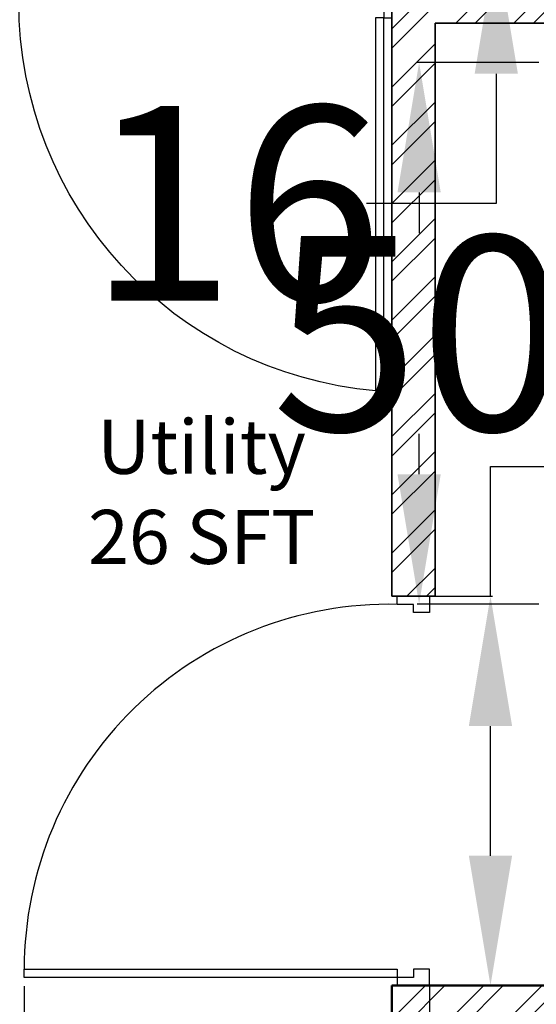
# Model space of a CAD drawing. Units: inches. Extents: x -90 to 536, y -553 to 299.
# Tile 3 of 27: x 49 to 96, y -430 to -339. Entities that reach past the tile are written whole.
import ezdxf

# ---------------------------------------------------------------- set-up
doc = ezdxf.new("R2010")
doc.units = ezdxf.units.IN
for name, color, linetype, lineweight in [('A-ANNO-DIMS', 2, 'Continuous', 18), ('A-AREA-IDEN', 7, 'Continuous', 18), ('A-DOOR', 4, 'Continuous', 25), ('A-WALL-PATT', 252, 'Continuous', 13), ('Inner Wall', 5, 'Continuous', 35), ('Outer Wall', 1, 'Continuous', 50)]:
    doc.layers.add(name, color=color, linetype=linetype, lineweight=lineweight)
doc.styles.get("Standard").update_dxf_attribs({"font": 'arial.ttf'})
doc.dimstyles.get("Standard").update_dxf_attribs({"dimtxt": 18, "dimasz": 12, "dimexe": 0.18, "dimexo": 0.0625, "dimgap": 0.09, "dimtad": 0, "dimtih": 1, "dimtoh": 1, "dimdec": 0, "dimzin": 0, "dimdsep": 46, "dimlunit": 3, "dimtxsty": 'Standard', "dimcen": 0.09, "dimadec": 0, "dimazin": 0, "dimtfac": 1, "dimtdec": 0, "dimtofl": 0, "dimtmove": 0, "dimatfit": 3, "dimfxl": 1, "dimtolj": 1, "dimtzin": 0, "dimarcsym": 0})

# ---------------------------------------------------------------- blocks, each defined once
blk = doc.blocks.new('DOOR-36-A')
for points in [[(35.25, 37.5), (35.25, 3), (34.5, 3), (34.5, 37.5)], [(0, 0), (1.5, 0), (1.5, 1.5), (0.75, 1.5), (0.75, 3), (0, 3)], [(36, 0), (34.5, 0), (34.5, 1.5), (35.25, 1.5), (35.25, 3), (36, 3)]]:
    blk.add_lwpolyline(points, close=True)
blk.add_arc((37.636, 1.5), 36.136, 94.97911, 180)
blk = doc.blocks.new('DOOR-36-B')
for points in [[(37.5, 36), (37.5, 34.5), (36, 34.5), (36, 35.25), (34.5, 35.25), (34.5, 36)], [(0, 0.75), (0, 1.5), (34.5, 1.5), (34.5, 0.75)], [(37.5, 0), (37.5, 1.5), (36, 1.5), (36, 0.75), (34.5, 0.75), (34.5, 0)]]:
    blk.add_lwpolyline(points, close=True)
blk.add_arc((33.758, 1.5), 33.758, 88.7408, 180)
blk = doc.blocks.new('*D27')
at = {"layer": 'A-ANNO-DIMS', "color": 0, "lineweight": -2, "transparency": 16777216}
for p, q in [((49.132, -428.616), (49.132, -434.359)), ((86.632, -428.616), (86.632, -434.359)), ((61.132, -434.179), (74.632, -434.179)), ((86.632, -434.179), (98.632, -434.179))]:
    blk.add_line(p, q, dxfattribs=at)
at = {"layer": 'A-ANNO-DIMS', "color": 0, "transparency": 16777216}
for points in [[(61.132, -432.179), (61.132, -436.179), (49.132, -434.179)], [(74.632, -432.179), (74.632, -436.179), (86.632, -434.179)]]:
    blk.add_solid(points, dxfattribs=at)
at = {"layer": 'Defpoints', "color": 0, "transparency": 16777216}
for p in [(49.132, -428.554), (86.632, -428.554), (86.632, -434.179)]:
    blk.add_point(p, dxfattribs=at)
at = {"layer": 'A-ANNO-DIMS', "color": 0, "transparency": 16777216, "insert": (195.174, -434.179), "char_height": 18, "attachment_point": 5}
blk.add_mtext('\\A1;DOOR B 38 TYP.', dxfattribs=at)
blk = doc.blocks.new('*D28')
at = {"layer": 'A-ANNO-DIMS', "color": 0, "lineweight": -2, "transparency": 16777216}
for p, q in [((92.257, -392.554), (92.257, -380.554)), ((92.257, -380.554), (104.257, -380.554)), ((86.694, -392.554), (92.437, -392.554)), ((92.257, -416.554), (92.257, -404.554)), ((86.694, -428.554), (92.437, -428.554))]:
    blk.add_line(p, q, dxfattribs=at)
at = {"layer": 'A-ANNO-DIMS', "color": 0, "transparency": 16777216}
for points in [[(90.257, -404.554), (94.257, -404.554), (92.257, -392.554)], [(90.257, -416.554), (94.257, -416.554), (92.257, -428.554)]]:
    blk.add_solid(points, dxfattribs=at)
at = {"layer": 'Defpoints', "color": 0, "transparency": 16777216}
for p in [(86.632, -392.554), (92.257, -392.554), (86.632, -428.554)]:
    blk.add_point(p, dxfattribs=at)
at = {"layer": 'A-ANNO-DIMS', "color": 0, "transparency": 16777216, "insert": (148.15, -380.554), "char_height": 18, "attachment_point": 5}
blk.add_mtext('\\A1;36 TYP.', dxfattribs=at)
blk = doc.blocks.new('*D46')
at = {"layer": 'A-ANNO-DIMS', "color": 0, "lineweight": -2, "transparency": 16777216}
for p, q in [((92.796, -304.194), (92.796, -292.194)), ((96.856, -316.194), (92.616, -316.194)), ((96.856, -332.226), (92.616, -332.226)), ((92.796, -344.226), (92.796, -356.226)), ((92.796, -356.226), (80.796, -356.226))]:
    blk.add_line(p, q, dxfattribs=at)
at = {"layer": 'A-ANNO-DIMS', "color": 0, "transparency": 16777216}
for points in [[(90.796, -304.194), (94.796, -304.194), (92.796, -316.194)], [(90.796, -344.226), (94.796, -344.226), (92.796, -332.226)]]:
    blk.add_solid(points, dxfattribs=at)
at = {"layer": 'Defpoints', "color": 0, "transparency": 16777216}
for p in [(96.919, -316.194), (92.796, -332.226), (96.919, -332.226)]:
    blk.add_point(p, dxfattribs=at)
at = {"layer": 'A-ANNO-DIMS', "color": 0, "transparency": 16777216, "insert": (68.667, -356.226), "char_height": 18, "attachment_point": 5}
blk.add_mtext('\\A1;16', dxfattribs=at)
blk = doc.blocks.new('*D52')
at = {"layer": 'A-ANNO-DIMS', "color": 0, "lineweight": -2, "transparency": 16777216}
for p, q in [((96.743, -343.206), (85.477, -343.206)), ((85.657, -355.206), (85.657, -358.961)), ((85.657, -381.277), (85.657, -377.522)), ((96.743, -393.277), (85.477, -393.277))]:
    blk.add_line(p, q, dxfattribs=at)
at = {"layer": 'A-ANNO-DIMS', "color": 0, "transparency": 16777216}
for points in [[(83.657, -355.206), (87.657, -355.206), (85.657, -343.206)], [(83.657, -381.277), (87.657, -381.277), (85.657, -393.277)]]:
    blk.add_solid(points, dxfattribs=at)
at = {"layer": 'Defpoints', "color": 0, "transparency": 16777216}
for p in [(96.806, -343.206), (85.657, -393.277), (96.806, -393.277)]:
    blk.add_point(p, dxfattribs=at)
at = {"layer": 'A-ANNO-DIMS', "color": 0, "transparency": 16777216, "insert": (85.657, -368.242), "char_height": 18, "attachment_point": 5}
blk.add_mtext('\\A1;50', dxfattribs=at)
blk = doc.blocks.new('*D54')
at = {"layer": 'A-ANNO-DIMS', "color": 0, "lineweight": -2, "transparency": 16777216}
for p, q in [((113.069, 249.446), (-2.848, 249.446)), ((-2.668, 237.446), (-2.668, -117.767)), ((-2.668, -491.554), (-2.668, -136.34)), ((38.069, -503.554), (-2.848, -503.554))]:
    blk.add_line(p, q, dxfattribs=at)
at = {"layer": 'A-ANNO-DIMS', "color": 0, "transparency": 16777216}
for points in [[(-4.668, 237.446), (-0.668, 237.446), (-2.668, 249.446)], [(-4.668, -491.554), (-0.668, -491.554), (-2.668, -503.554)]]:
    blk.add_solid(points, dxfattribs=at)
at = {"layer": 'Defpoints', "color": 0, "transparency": 16777216}
for p in [(-2.668, 249.446), (113.132, 249.446), (38.132, -503.554)]:
    blk.add_point(p, dxfattribs=at)
at = {"layer": 'A-ANNO-DIMS', "color": 0, "transparency": 16777216, "insert": (-2.668, -127.054), "char_height": 18, "attachment_point": 5}
blk.add_mtext('\\A1;753', dxfattribs=at)

msp = doc.modelspace()

# ---------------------------------------------------------------- hatches: boundary and pattern name
at = {"layer": 'A-WALL-PATT'}
h = msp.add_hatch(dxfattribs=at)
h.set_pattern_fill('ANSI32', color=256, scale=0.4)
h.set_pattern_definition([(45, (-88.8105, -603.6155), (-2.694077, 2.694077), []), (45, (-87.0145, -603.6155), (-2.694077, 2.694077), [])])
h.paths.add_polyline_path([(285.1317, 246.4462), (131.1317, 246.4462), (131.1317, 237.4462), (285.1317, 237.4462)])
h.paths.add_polyline_path([(122.1317, 237.4462), (113.1317, 237.4462), (113.1317, 152.4462), (122.1317, 152.4462), (122.1317, 166.4704)])
h.paths.add_polyline_path([(303.1317, 237.4462), (294.1317, 237.4462), (294.1317, 152.4462), (303.1317, 152.4462)])
h.paths.add_polyline_path([(47.1317, 91.9277), (38.1317, 91.9277), (38.1317, -6.5538), (77.1317, -6.5538), (77.1317, 2.4462), (70.5655, 2.4462), (47.1317, 2.4462)])
h.paths.add_polyline_path([(83.052, -61.5538), (47.1317, -61.5538), (47.1317, -24.5538), (38.1317, -24.5538), (38.1317, -70.5538), (74.052, -70.5538), (74.052, -223.5538), (38.1317, -223.5538), (38.1317, -503.5538), (92.1317, -503.5538), (92.1317, -437.5538), (191.1317, -437.5538), (191.1317, -428.5538), (83.1317, -428.5538), (83.1317, -494.5538), (47.1317, -494.5538), (47.1317, -232.5538), (83.052, -232.5538), (83.052, -70.5538)])
h.paths.add_polyline_path([(407.1317, -63.5538), (381.1317, -63.5538), (381.1317, 91.9277), (372.1317, 91.9277), (372.1317, 32.8805), (372.1317, -63.5538), (306.5745, -63.5538), (237.1317, -63.5538), (237.1317, -38.5538), (233.1317, -38.5538), (233.1317, -71.5538), (398.1317, -71.5538), (398.1317, -152.5538), (233.1317, -152.5538), (233.1317, -161.5538), (398.1317, -161.5538), (398.1317, -368.5538), (233.1317, -368.5538), (233.1317, -377.5538), (407.1317, -377.5538), (407.1317, -161.5538)])
h.paths.add_polyline_path([(261.1317, -422.5538), (252.1317, -422.5538), (252.1317, -428.5538), (233.1317, -428.5538), (233.1317, -437.5538), (261.1317, -437.5538)])
h.paths.add_polyline_path([(191.1317, -368.5538), (180.1317, -368.5538), (180.1317, -335.5538), (131.5919, -335.5538), (131.5919, -344.5538), (171.1317, -344.5538), (171.1317, -392.5538), (180.1317, -392.5538), (180.1317, -377.5538), (191.1317, -377.5538)], flags=17)
h.paths.add_polyline_path([(180.1317, -223.5538), (152.1317, -223.5538), (152.1317, -227.5538), (176.1317, -227.5538), (176.1317, -335.5538), (180.1317, -335.5538)], flags=17)
h.paths.add_polyline_path([(131.5919, -335.5538), (83.1317, -335.5538), (83.1317, -339.5538), (83.1317, -392.5538), (87.1317, -392.5538), (87.1317, -339.5538), (131.5919, -339.5538)], flags=17)
h.paths.add_polyline_path([(197.1317, 2.4462), (77.1317, 2.4462), (77.1317, -1.5538), (113.1317, -1.5538), (113.1317, -71.5538), (181.1317, -71.5538), (181.1317, -67.5538), (117.1317, -67.5538), (117.1317, -1.5538), (177.1317, -1.5538), (177.1317, -37.5538), (181.1317, -37.5538), (181.1317, -1.5538), (197.1317, -1.5538)])
h.paths.add_polyline_path([(173.1317, 138.4462), (122.1317, 138.4462), (122.1317, 134.4462), (173.1317, 134.4462)])
h.paths.add_polyline_path([(213.1317, 237.4462), (209.1317, 237.4462), (209.1317, 134.4462), (233.1317, 134.4462), (233.1317, 68.8889), (233.1317, -2.5538), (237.1317, -2.5538), (237.1317, 134.4462), (258.1317, 134.4462), (258.1317, 138.4462), (213.1317, 138.4462)])

# ---------------------------------------------------------------- linework, layer by layer
at = {"layer": 'Inner Wall'}
for p, q in [((83.1317, -339.5538), (83.1317, -335.5538)), ((83.1317, -339.5538), (83.1317, -392.5538)), ((87.1317, -339.5538), (131.5919, -339.5538)), ((87.1317, -339.5538), (87.1317, -392.5538)), ((87.1317, -392.5538), (83.1317, -392.5538))]:
    msp.add_line(p, q, dxfattribs=at)
at = {"layer": 'Outer Wall'}
for p, q in [((191.1317, -428.5538), (83.1317, -428.5538)), ((83.1317, -428.5538), (83.1317, -494.5538))]:
    msp.add_line(p, q, dxfattribs=at)

# ---------------------------------------------------------------- block references
at = {"layer": 'A-DOOR', "extrusion": (0, 0, -1), "zscale": -1, "rotation": 180}
msp.add_blockref('DOOR-36-A', (-47.1317, -336.0538), dxfattribs=at)
at = {"layer": 'A-DOOR'}
msp.add_blockref('DOOR-36-B', (49.1317, -428.5538), dxfattribs=at)

# ---------------------------------------------------------------- texts
at = {"layer": 'A-AREA-IDEN', "insert": (90.2088, -376.2326), "char_height": 5, "attachment_point": 3}
msp.add_mtext_dynamic_manual_height_columns('\\pxqc;{\\fTimes New Roman|b0|i0|c0|p18;Utility\\P26 SFT}', width=49.342153, gutter_width=12.5, heights=[0], dxfattribs=at)

# ---------------------------------------------------------------- dimensions: what is measured, and where the dimension line sits
at = {"layer": 'A-ANNO-DIMS'}
for base, p1, p2, angle, picture, middle in [((-2.6677, 249.4462), (38.1317, -503.5538), (113.1317, 249.4462), 90, '*D54', (-2.6677, -127.0538)), ((92.7963, -332.2258), (96.9187, -316.194), (96.9187, -332.2258), 270, '*D46', (68.6674, -356.2258)), ((85.6567, -393.2773), (96.8056, -343.2061), (96.8056, -393.2773), 270, '*D52', (85.6567, -368.2417))]:
    dim = msp.add_linear_dim(base=base, p1=p1, p2=p2, angle=angle, dimstyle='Standard', override={"dimdec": 0, "dimlfac": 1, "dimrnd": 0, "dimzin": 0, "dimdsep": 46, "dimlunit": 2}, dxfattribs=at)
    dim.commit()
    dim.dimension.update_dxf_attribs({"geometry": picture, "text_midpoint": middle})
dim = msp.add_linear_dim(base=(92.2567, -392.5538), p1=(86.6317, -428.5538), p2=(86.6317, -392.5538), angle=90, text='<> TYP.', dimstyle='Standard', override={"dimdec": 0, "dimlfac": 1, "dimrnd": 0, "dimzin": 0, "dimdsep": 46, "dimlunit": 2}, dxfattribs=at)
dim.commit()
dim.dimension.update_dxf_attribs({"geometry": '*D28', "text_midpoint": (148.1496, -380.5538)})
dim = msp.add_linear_dim(base=(86.6317404714, -434.1787825705), p1=(49.1317404714, -428.5537825705), p2=(86.6317404714, -428.5537825705), text='DOOR B <> TYP.', dimstyle='Standard', override={"dimdec": 0, "dimlfac": 1, "dimrnd": 0, "dimzin": 0, "dimdsep": 46, "dimlunit": 2}, dxfattribs=at)
dim.commit()
dim.dimension.update_dxf_attribs({"geometry": '*D27', "text_midpoint": (195.1739914946, -434.1787825705)})

doc.saveas('drawing.dxf')
